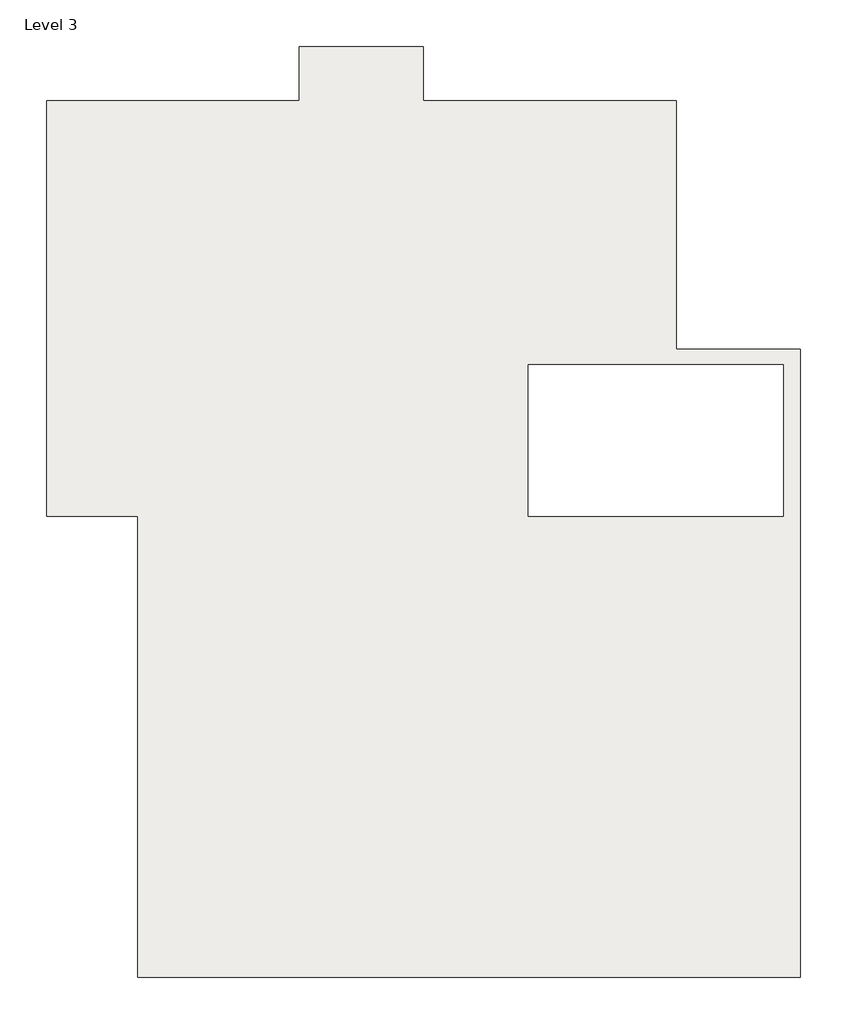
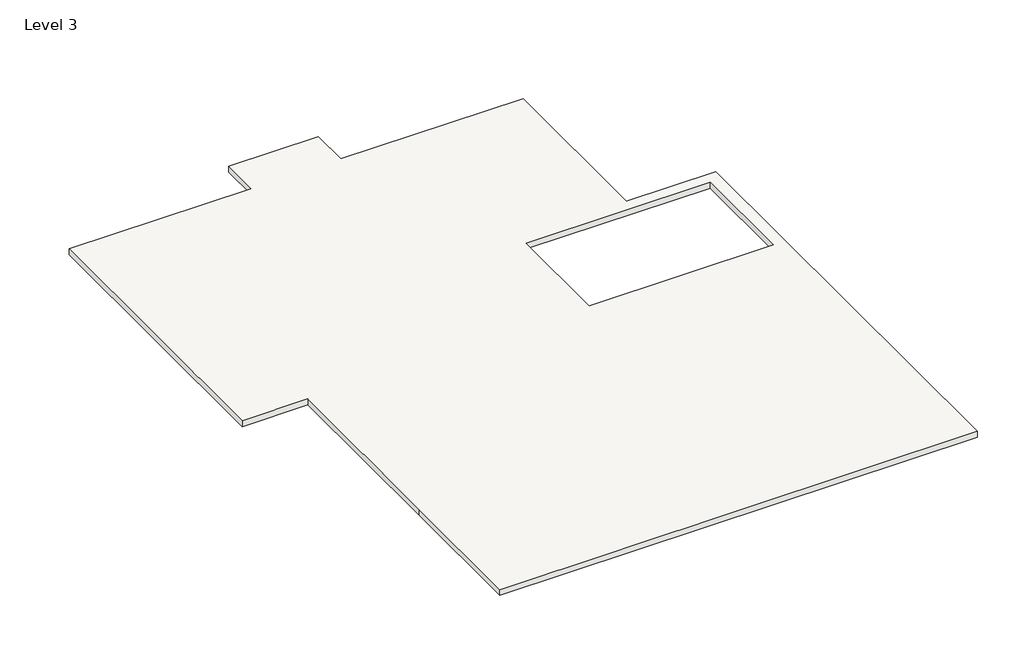
# One storey: 1 slab.
"""IFC4 building model written with IfcOpenShell, lengths in millimetres."""

from ifc_helpers import new_model, si_unit, frame, origin, place, context, project, spatial, polyline, outline, extrude, element, save

model = new_model("IFC4")

# Units and contexts
model_context = context("Model", 3, world=origin())
ifc_project = project(units=[si_unit("LENGTHUNIT", "METRE", prefix="MILLI")], contexts=[model_context])

# Site, building, storey
site = spatial("IfcSite", under=ifc_project)
building = spatial("IfcBuilding", under=site)
storey = spatial("IfcBuildingStorey", under=building, Name="Level 3", Elevation=6400.8)

# Slab
placement = place(None, origin())
element("IfcSlab", 1, ObjectType="Generic - 6\"", at=placement, inside=storey, context=model_context, shape_type="SweptSolid", body=[
    extrude(outline(polyline([(-8486.2183666, 3612.3503619), (-8486.2183666, -7563.6496381), (-20271.8183666, -7563.6496381), (-20271.8183666, -4118.4260556), (-20271.8183666, 640.5503619), (-21897.4183666, 640.5503619), (-21897.4183666, 8031.9503619), (-17401.6183666, 8031.9503619), (-17401.6183666, 8997.1503619), (-15191.8183666, 8997.1503619), (-15191.8183666, 8031.9503619), (-10696.0183666, 8031.9503619), (-10696.0183666, 3612.3503619), (-8486.2183666, 3612.3503619)]), holes=[polyline([(-13326.4629678, 3332.9503619), (-13326.4629678, 640.5503619), (-8791.0183666, 640.5503619), (-8791.0183666, 3332.9503619), (-13326.4629678, 3332.9503619)])]), frame((0.0, 0.0, 6680.2), z_axis=(0.0, 0.0, 1.0), x_axis=(1.0, 0.0, 0.0)), (0.0, 0.0, 1.0), 152.4),
])

save(model, "model.ifc")

# Revit data of these elements
# Type "Generic - 6\""
#   Assembly Code = "B1010"
#   Function = 0
#   Layers, outside or top first: 0' - 6" no material (function 1)
# Element 1 (IfcSlab, "Generic - 6\"")
#   built-in parameter 1001955 = 1.5708 (stored number, unit not read)
#   Height Offset From Level = 1' - 5"
#   Phase Created = New Construction
#   Materials on its faces: "Default Floor"
# Materials
#   "Default Floor": colour RGB 128 128 128, transparency 0, Cost = 0
